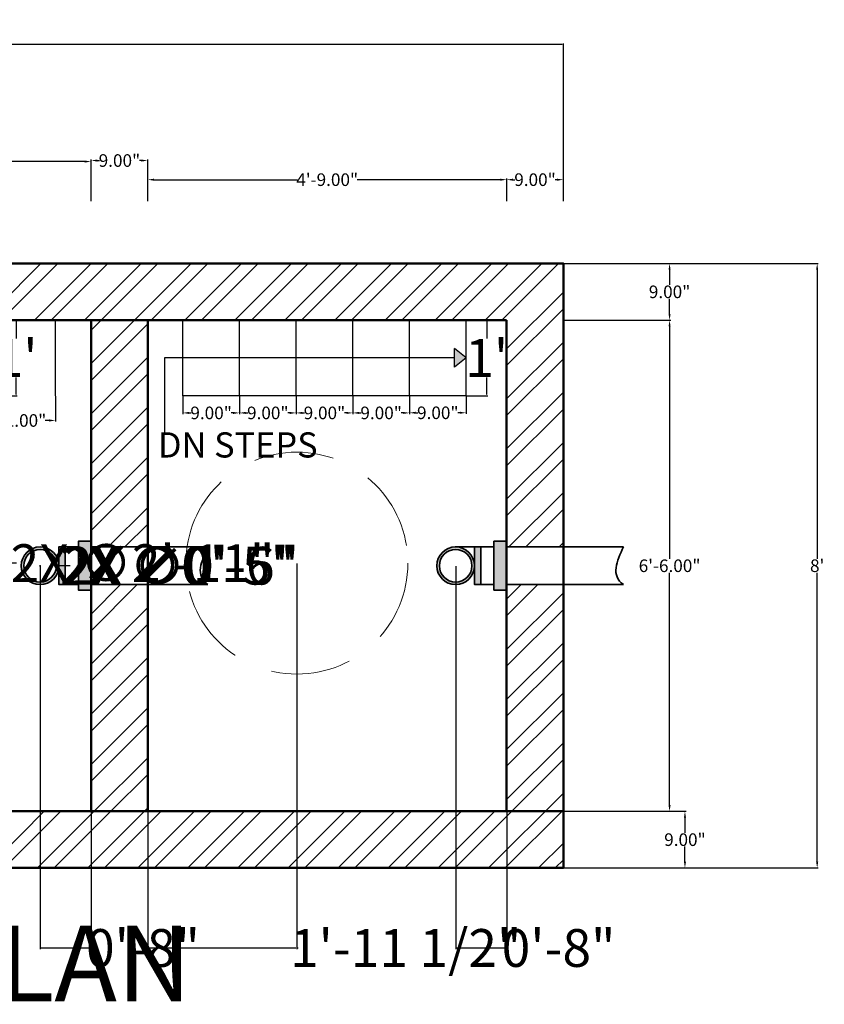
# Model space of a CAD drawing. Units: inches. Extents: x -34 to 285, y -151 to 155.
# Tile 10 of 10: x 129 to 256, y -2 to 155. Entities that reach past the tile are written whole.
import ezdxf

# ---------------------------------------------------------------- set-up
doc = ezdxf.new("R2010")
doc.units = ezdxf.units.IN
doc.header["$MEASUREMENT"] = 0
doc.linetypes.add('DASHED', pattern=[19.05, 12.7, -6.35])
for name, color, linetype, lineweight in [('A-ANNO-DIMS', 2, 'Continuous', 18), ('A-ANNO-TEXT', 7, 'Continuous', 25), ('A-DETL-HIDN', 8, 'DASHED', 18), ('A-FLOR-STRS', 3, 'Continuous', 25), ('A-WALL', 7, 'Continuous', 50), ('A-WALL-PATT', 8, 'Continuous', 18), ('P-SANR-PIPE', 4, 'Continuous', 35)]:
    doc.layers.add(name, color=color, linetype=linetype, lineweight=lineweight)
doc.styles.get("Standard").update_dxf_attribs({"font": 'arial.ttf'})
doc.dimstyles.get("Standard").update_dxf_attribs({"dimtxt": 6, "dimasz": 0.18, "dimexe": 0.18, "dimexo": 0.0625, "dimgap": 0.09, "dimtad": 0, "dimtih": 1, "dimtoh": 1, "dimzin": 0, "dimdsep": 46, "dimlunit": 3, "dimtxsty": 'Standard', "dimcen": 0.09, "dimadec": 0, "dimazin": 0, "dimtfac": 1, "dimtofl": 0, "dimtmove": 0, "dimatfit": 3, "dimfxl": 1, "dimtolj": 1, "dimtzin": 0, "dimarcsym": 0})

# ---------------------------------------------------------------- blocks, each defined once
blk = doc.blocks.new('*D1')
at = {"layer": 'A-ANNO-DIMS', "color": 0, "lineweight": -2, "transparency": 16777216}
for p, q in [((199.47, 106.98), (202.86, 106.98)), ((202.68, 106.8), (202.68, 104.08)), ((202.68, 95.16), (202.68, 97.88)), ((199.47, 94.98), (202.86, 94.98))]:
    blk.add_line(p, q, dxfattribs=at)
at = {"layer": 'A-ANNO-DIMS', "color": 0, "transparency": 16777216}
for points in [[(202.65, 106.8), (202.71, 106.8), (202.68, 106.98)], [(202.65, 95.16), (202.71, 95.16), (202.68, 94.98)]]:
    blk.add_solid(points, dxfattribs=at)
at = {"layer": 'Defpoints', "color": 0, "transparency": 16777216}
for p in [(199.41, 106.98), (199.41, 94.98), (202.68, 94.98)]:
    blk.add_point(p, dxfattribs=at)
at = {"layer": 'A-ANNO-DIMS', "color": 0, "transparency": 16777216, "insert": (202.68, 100.98), "char_height": 6, "attachment_point": 5}
blk.add_mtext("\\A1;1'", dxfattribs=at)
blk = doc.blocks.new('*D2')
at = {"layer": 'A-ANNO-DIMS', "color": 0, "lineweight": -2, "transparency": 16777216}
for p, q in [((190.41, 94.92), (190.41, 92.09)), ((199.41, 94.92), (199.41, 92.09)), ((191.41, 92.27), (191.73, 92.27)), ((198.41, 92.27), (198.09, 92.27))]:
    blk.add_line(p, q, dxfattribs=at)
at = {"layer": 'A-ANNO-DIMS', "color": 0, "transparency": 16777216}
for points in [[(191.41, 92.44), (191.41, 92.11), (190.41, 92.27)], [(198.41, 92.44), (198.41, 92.11), (199.41, 92.27)]]:
    blk.add_solid(points, dxfattribs=at)
at = {"layer": 'Defpoints', "color": 0, "transparency": 16777216}
for p in [(190.41, 94.98), (199.41, 94.98), (199.41, 92.27)]:
    blk.add_point(p, dxfattribs=at)
at = {"layer": 'A-ANNO-DIMS', "color": 0, "transparency": 16777216, "insert": (194.91, 92.27), "char_height": 2, "attachment_point": 5}
blk.add_mtext('\\A1;9.00"', dxfattribs=at)
blk = doc.blocks.new('*D3')
at = {"layer": 'A-ANNO-DIMS', "color": 0, "lineweight": -2, "transparency": 16777216}
for p, q in [((181.41, 94.92), (181.41, 92.07)), ((190.41, 94.92), (190.41, 92.07)), ((182.41, 92.25), (182.73, 92.25)), ((189.41, 92.25), (189.09, 92.25))]:
    blk.add_line(p, q, dxfattribs=at)
at = {"layer": 'A-ANNO-DIMS', "color": 0, "transparency": 16777216}
for points in [[(182.41, 92.41), (182.41, 92.08), (181.41, 92.25)], [(189.41, 92.41), (189.41, 92.08), (190.41, 92.25)]]:
    blk.add_solid(points, dxfattribs=at)
at = {"layer": 'Defpoints', "color": 0, "transparency": 16777216}
for p in [(181.41, 94.98), (190.41, 94.98), (181.41, 92.25)]:
    blk.add_point(p, dxfattribs=at)
at = {"layer": 'A-ANNO-DIMS', "color": 0, "transparency": 16777216, "insert": (185.91, 92.25), "char_height": 2, "attachment_point": 5}
blk.add_mtext('\\A1;9.00"', dxfattribs=at)
blk = doc.blocks.new('*D4')
at = {"layer": 'A-ANNO-DIMS', "color": 0, "lineweight": -2, "transparency": 16777216}
for p, q in [((172.41, 94.92), (172.41, 92.07)), ((181.41, 94.92), (181.41, 92.07)), ((173.41, 92.25), (173.73, 92.25)), ((180.41, 92.25), (180.09, 92.25))]:
    blk.add_line(p, q, dxfattribs=at)
at = {"layer": 'A-ANNO-DIMS', "color": 0, "transparency": 16777216}
for points in [[(173.41, 92.41), (173.41, 92.08), (172.41, 92.25)], [(180.41, 92.41), (180.41, 92.08), (181.41, 92.25)]]:
    blk.add_solid(points, dxfattribs=at)
at = {"layer": 'Defpoints', "color": 0, "transparency": 16777216}
for p in [(172.41, 94.98), (181.41, 94.98), (172.41, 92.25)]:
    blk.add_point(p, dxfattribs=at)
at = {"layer": 'A-ANNO-DIMS', "color": 0, "transparency": 16777216, "insert": (176.91, 92.25), "char_height": 2, "attachment_point": 5}
blk.add_mtext('\\A1;9.00"', dxfattribs=at)
blk = doc.blocks.new('*D5')
at = {"layer": 'A-ANNO-DIMS', "color": 0, "lineweight": -2, "transparency": 16777216}
for p, q in [((163.41, 94.92), (163.41, 92.07)), ((172.41, 94.92), (172.41, 92.07)), ((164.41, 92.25), (164.73, 92.25)), ((171.41, 92.25), (171.09, 92.25))]:
    blk.add_line(p, q, dxfattribs=at)
at = {"layer": 'A-ANNO-DIMS', "color": 0, "transparency": 16777216}
for points in [[(164.41, 92.41), (164.41, 92.08), (163.41, 92.25)], [(171.41, 92.41), (171.41, 92.08), (172.41, 92.25)]]:
    blk.add_solid(points, dxfattribs=at)
at = {"layer": 'Defpoints', "color": 0, "transparency": 16777216}
for p in [(163.41, 94.98), (172.41, 94.98), (163.41, 92.25)]:
    blk.add_point(p, dxfattribs=at)
at = {"layer": 'A-ANNO-DIMS', "color": 0, "transparency": 16777216, "insert": (167.91, 92.25), "char_height": 2, "attachment_point": 5}
blk.add_mtext('\\A1;9.00"', dxfattribs=at)
blk = doc.blocks.new('*D6')
at = {"layer": 'A-ANNO-DIMS', "color": 0, "lineweight": -2, "transparency": 16777216}
for p, q in [((154.41, 94.92), (154.41, 92.07)), ((163.41, 94.92), (163.41, 92.07)), ((155.41, 92.25), (155.73, 92.25)), ((162.41, 92.25), (162.09, 92.25))]:
    blk.add_line(p, q, dxfattribs=at)
at = {"layer": 'A-ANNO-DIMS', "color": 0, "transparency": 16777216}
for points in [[(155.41, 92.41), (155.41, 92.08), (154.41, 92.25)], [(162.41, 92.41), (162.41, 92.08), (163.41, 92.25)]]:
    blk.add_solid(points, dxfattribs=at)
at = {"layer": 'Defpoints', "color": 0, "transparency": 16777216}
for p in [(154.41, 94.98), (163.41, 94.98), (154.41, 92.25)]:
    blk.add_point(p, dxfattribs=at)
at = {"layer": 'A-ANNO-DIMS', "color": 0, "transparency": 16777216, "insert": (158.91, 92.25), "char_height": 2, "attachment_point": 5}
blk.add_mtext('\\A1;9.00"', dxfattribs=at)
blk = doc.blocks.new('*D7')
at = {"layer": 'A-ANNO-DIMS', "color": 0, "lineweight": -2, "transparency": 16777216}
for p, q in [((123.25, 106.98), (128.12, 106.98)), ((127.94, 106.8), (127.94, 104.08)), ((127.94, 95.16), (127.94, 97.88)), ((123.25, 94.98), (128.12, 94.98))]:
    blk.add_line(p, q, dxfattribs=at)
at = {"layer": 'A-ANNO-DIMS', "color": 0, "transparency": 16777216}
for points in [[(127.91, 106.8), (127.97, 106.8), (127.94, 106.98)], [(127.91, 95.16), (127.97, 95.16), (127.94, 94.98)]]:
    blk.add_solid(points, dxfattribs=at)
at = {"layer": 'Defpoints', "color": 0, "transparency": 16777216}
for p in [(123.18, 106.98), (123.18, 94.98), (127.94, 94.98)]:
    blk.add_point(p, dxfattribs=at)
at = {"layer": 'A-ANNO-DIMS', "color": 0, "transparency": 16777216, "insert": (127.94, 100.98), "char_height": 6, "attachment_point": 5}
blk.add_mtext("\\A1;1'", dxfattribs=at)
blk = doc.blocks.new('*D13')
at = {"layer": 'A-ANNO-DIMS', "color": 0, "lineweight": -2, "transparency": 16777216}
for p, q in [((123.18, 94.92), (123.18, 90.87)), ((134.18, 94.92), (134.18, 90.87)), ((124.18, 91.05), (124.82, 91.05)), ((133.18, 91.05), (132.55, 91.05))]:
    blk.add_line(p, q, dxfattribs=at)
at = {"layer": 'A-ANNO-DIMS', "color": 0, "transparency": 16777216}
for points in [[(124.18, 91.22), (124.18, 90.88), (123.18, 91.05)], [(133.18, 91.22), (133.18, 90.88), (134.18, 91.05)]]:
    blk.add_solid(points, dxfattribs=at)
at = {"layer": 'Defpoints', "color": 0, "transparency": 16777216}
for p in [(123.18, 94.98), (134.18, 94.98), (134.18, 91.05)]:
    blk.add_point(p, dxfattribs=at)
at = {"layer": 'A-ANNO-DIMS', "color": 0, "transparency": 16777216, "insert": (128.68, 91.05), "char_height": 2, "attachment_point": 5}
blk.add_mtext('\\A1;11.00"', dxfattribs=at)
blk = doc.blocks.new('*D17')
at = {"layer": 'A-ANNO-DIMS', "color": 0, "lineweight": -2, "transparency": 16777216}
for p, q in [((70.85, 125.9), (70.85, 132.35)), ((71.85, 132.17), (100.66, 132.17)), ((138.85, 132.17), (110.04, 132.17)), ((139.85, 125.9), (139.85, 132.35))]:
    blk.add_line(p, q, dxfattribs=at)
at = {"layer": 'A-ANNO-DIMS', "color": 0, "transparency": 16777216}
for points in [[(71.85, 132.33), (71.85, 132), (70.85, 132.17)], [(138.85, 132.33), (138.85, 132), (139.85, 132.17)]]:
    blk.add_solid(points, dxfattribs=at)
at = {"layer": 'Defpoints', "color": 0, "transparency": 16777216}
for p in [(139.85, 132.17), (70.85, 125.83), (139.85, 125.83)]:
    blk.add_point(p, dxfattribs=at)
at = {"layer": 'A-ANNO-DIMS', "color": 0, "transparency": 16777216, "insert": (105.35, 132.17), "char_height": 2, "attachment_point": 5}
blk.add_mtext('\\A1;5\'-9.00"', dxfattribs=at)
blk = doc.blocks.new('*D18')
at = {"layer": 'A-ANNO-DIMS', "color": 0, "lineweight": -2, "transparency": 16777216}
for p, q in [((139.85, 125.9), (139.85, 132.51)), ((140.85, 132.33), (141.16, 132.33)), ((147.85, 132.33), (147.53, 132.33)), ((148.85, 125.9), (148.85, 132.51))]:
    blk.add_line(p, q, dxfattribs=at)
at = {"layer": 'A-ANNO-DIMS', "color": 0, "transparency": 16777216}
for points in [[(140.85, 132.49), (140.85, 132.16), (139.85, 132.33)], [(147.85, 132.49), (147.85, 132.16), (148.85, 132.33)]]:
    blk.add_solid(points, dxfattribs=at)
at = {"layer": 'Defpoints', "color": 0, "transparency": 16777216}
for p in [(148.85, 132.33), (139.85, 125.83), (148.85, 125.83)]:
    blk.add_point(p, dxfattribs=at)
at = {"layer": 'A-ANNO-DIMS', "color": 0, "transparency": 16777216, "insert": (144.35, 132.33), "char_height": 2, "attachment_point": 5}
blk.add_mtext('\\A1;9.00"', dxfattribs=at)
blk = doc.blocks.new('*D19')
at = {"layer": 'A-ANNO-DIMS', "color": 0, "lineweight": -2, "transparency": 16777216}
for p, q in [((148.85, 125.9), (148.85, 129.47)), ((149.85, 129.29), (172.62, 129.29)), ((204.85, 129.29), (182.08, 129.29)), ((205.85, 125.9), (205.85, 129.47))]:
    blk.add_line(p, q, dxfattribs=at)
at = {"layer": 'A-ANNO-DIMS', "color": 0, "transparency": 16777216}
for points in [[(149.85, 129.45), (149.85, 129.12), (148.85, 129.29)], [(204.85, 129.45), (204.85, 129.12), (205.85, 129.29)]]:
    blk.add_solid(points, dxfattribs=at)
at = {"layer": 'Defpoints', "color": 0, "transparency": 16777216}
for p in [(205.85, 129.29), (148.85, 125.83), (205.85, 125.83)]:
    blk.add_point(p, dxfattribs=at)
at = {"layer": 'A-ANNO-DIMS', "color": 0, "transparency": 16777216, "insert": (177.35, 129.29), "char_height": 2, "attachment_point": 5}
blk.add_mtext('\\A1;4\'-9.00"', dxfattribs=at)
blk = doc.blocks.new('*D20')
at = {"layer": 'A-ANNO-DIMS', "color": 0, "lineweight": -2, "transparency": 16777216}
for p, q in [((205.85, 125.9), (205.85, 129.47)), ((206.85, 129.29), (207.16, 129.29)), ((213.85, 129.29), (213.53, 129.29)), ((214.85, 125.9), (214.85, 129.47))]:
    blk.add_line(p, q, dxfattribs=at)
at = {"layer": 'A-ANNO-DIMS', "color": 0, "transparency": 16777216}
for points in [[(206.85, 129.45), (206.85, 129.12), (205.85, 129.29)], [(213.85, 129.45), (213.85, 129.12), (214.85, 129.29)]]:
    blk.add_solid(points, dxfattribs=at)
at = {"layer": 'Defpoints', "color": 0, "transparency": 16777216}
for p in [(214.85, 129.29), (205.85, 125.83), (214.85, 125.83)]:
    blk.add_point(p, dxfattribs=at)
at = {"layer": 'A-ANNO-DIMS', "color": 0, "transparency": 16777216, "insert": (210.35, 129.29), "char_height": 2, "attachment_point": 5}
blk.add_mtext('\\A1;9.00"', dxfattribs=at)
blk = doc.blocks.new('*D21')
at = {"layer": 'A-ANNO-DIMS', "color": 0, "lineweight": -2, "transparency": 16777216}
for p, q in [((22.85, 130.62), (22.85, 150.94)), ((23.03, 150.76), (113.95, 150.76)), ((214.67, 150.76), (123.74, 150.76)), ((214.85, 127.74), (214.85, 150.94))]:
    blk.add_line(p, q, dxfattribs=at)
at = {"layer": 'A-ANNO-DIMS', "color": 0, "transparency": 16777216}
for points in [[(23.03, 150.79), (23.03, 150.73), (22.85, 150.76)], [(214.67, 150.79), (214.67, 150.73), (214.85, 150.76)]]:
    blk.add_solid(points, dxfattribs=at)
at = {"layer": 'Defpoints', "color": 0, "transparency": 16777216}
for p in [(22.85, 150.76), (22.85, 130.55), (214.85, 127.68)]:
    blk.add_point(p, dxfattribs=at)
at = {"layer": 'A-ANNO-DIMS', "color": 0, "transparency": 16777216, "insert": (118.85, 150.76), "char_height": 6, "attachment_point": 5}
blk.add_mtext("\\A1;16'", dxfattribs=at)
blk = doc.blocks.new('*D22')
at = {"layer": 'A-ANNO-DIMS', "color": 0, "lineweight": -2, "transparency": 16777216}
for p, q in [((214.91, 115.98), (231.9, 115.98)), ((231.72, 114.98), (231.72, 112.59)), ((231.72, 107.98), (231.72, 110.37)), ((214.91, 106.98), (231.9, 106.98))]:
    blk.add_line(p, q, dxfattribs=at)
at = {"layer": 'A-ANNO-DIMS', "color": 0, "transparency": 16777216}
for points in [[(231.55, 114.98), (231.88, 114.98), (231.72, 115.98)], [(231.55, 107.98), (231.88, 107.98), (231.72, 106.98)]]:
    blk.add_solid(points, dxfattribs=at)
at = {"layer": 'Defpoints', "color": 0, "transparency": 16777216}
for p in [(214.85, 115.98), (231.72, 115.98), (214.85, 106.98)]:
    blk.add_point(p, dxfattribs=at)
at = {"layer": 'A-ANNO-DIMS', "color": 0, "transparency": 16777216, "insert": (231.72, 111.48), "char_height": 2, "attachment_point": 5}
blk.add_mtext('\\A1;9.00"', dxfattribs=at)
blk = doc.blocks.new('*D23')
at = {"layer": 'A-ANNO-DIMS', "color": 0, "lineweight": -2, "transparency": 16777216}
for p, q in [((214.91, 28.98), (234.34, 28.98)), ((234.16, 27.98), (234.16, 25.59)), ((234.16, 20.98), (234.16, 23.37)), ((214.91, 19.98), (234.34, 19.98))]:
    blk.add_line(p, q, dxfattribs=at)
at = {"layer": 'A-ANNO-DIMS', "color": 0, "transparency": 16777216}
for points in [[(234, 27.98), (234.33, 27.98), (234.16, 28.98)], [(234, 20.98), (234.33, 20.98), (234.16, 19.98)]]:
    blk.add_solid(points, dxfattribs=at)
at = {"layer": 'Defpoints', "color": 0, "transparency": 16777216}
for p in [(214.85, 28.98), (214.85, 19.98), (234.16, 19.98)]:
    blk.add_point(p, dxfattribs=at)
at = {"layer": 'A-ANNO-DIMS', "color": 0, "transparency": 16777216, "insert": (234.16, 24.48), "char_height": 2, "attachment_point": 5}
blk.add_mtext('\\A1;9.00"', dxfattribs=at)
blk = doc.blocks.new('*D24')
at = {"layer": 'A-ANNO-DIMS', "color": 0, "lineweight": -2, "transparency": 16777216}
for p, q in [((231.78, 106.98), (231.9, 106.98)), ((231.72, 105.98), (231.72, 69.09)), ((231.72, 29.98), (231.72, 66.87)), ((231.78, 28.98), (231.9, 28.98))]:
    blk.add_line(p, q, dxfattribs=at)
at = {"layer": 'A-ANNO-DIMS', "color": 0, "transparency": 16777216}
for points in [[(231.55, 105.98), (231.88, 105.98), (231.72, 106.98)], [(231.55, 29.98), (231.88, 29.98), (231.72, 28.98)]]:
    blk.add_solid(points, dxfattribs=at)
at = {"layer": 'Defpoints', "color": 0, "transparency": 16777216}
for p in [(231.72, 106.98), (231.72, 28.98), (231.72, 28.98)]:
    blk.add_point(p, dxfattribs=at)
at = {"layer": 'A-ANNO-DIMS', "color": 0, "transparency": 16777216, "insert": (231.72, 67.98), "char_height": 2, "attachment_point": 5}
blk.add_mtext('\\A1;6\'-6.00"', dxfattribs=at)
blk = doc.blocks.new('*D25')
at = {"layer": 'A-ANNO-DIMS', "color": 0, "lineweight": -2, "transparency": 16777216}
for p, q in [((231.96, 115.98), (255.34, 115.98)), ((255.16, 114.98), (255.16, 69.09)), ((255.16, 20.98), (255.16, 66.87)), ((231.78, 19.98), (255.34, 19.98))]:
    blk.add_line(p, q, dxfattribs=at)
at = {"layer": 'A-ANNO-DIMS', "color": 0, "transparency": 16777216}
for points in [[(254.99, 114.98), (255.32, 114.98), (255.16, 115.98)], [(254.99, 20.98), (255.32, 20.98), (255.16, 19.98)]]:
    blk.add_solid(points, dxfattribs=at)
at = {"layer": 'Defpoints', "color": 0, "transparency": 16777216}
for p in [(231.9, 115.98), (255.16, 115.98), (231.72, 19.98)]:
    blk.add_point(p, dxfattribs=at)
at = {"layer": 'A-ANNO-DIMS', "color": 0, "transparency": 16777216, "insert": (255.16, 67.98), "char_height": 2, "attachment_point": 5}
blk.add_mtext("\\A1;8'", dxfattribs=at)
blk = doc.blocks.new('PIPE-BEND-PLAN')
h = blk.add_hatch(color=256)
h.dxf.hatch_style = 1
h.paths.add_polyline_path([(3.06, 6.87), (2.93, 6.87, 0.408167), (0, 3.87, 1), (5.99, 3.87, 0.408167)])
h.paths.add_polyline_path([(5.59, 3.87, -1), (0.4, 3.87, -1)], flags=16)
h = blk.add_hatch(color=256)
h.dxf.hatch_style = 1
h.paths.add_polyline_path([(6.97, 6.87), (5.99, 6.87), (5.99, 0.87), (6.97, 0.87)])
h = blk.add_hatch(color=256)
h.dxf.hatch_style = 1
h.paths.add_polyline_path([(11.09, 7.75), (9.08, 7.75), (9.08, 0), (11.09, 0)])
for points in [[(6.97, 6.88), (5.99, 6.88), (5.99, 0.87), (6.97, 0.87)], [(9.08, 6.88), (6.97, 6.88), (6.97, 0.87), (9.08, 0.87)], [(11.09, 7.75), (9.08, 7.75), (9.08, 0), (11.09, 0)]]:
    blk.add_lwpolyline(points, close=True)
for radius in [2.99, 2.59]:
    blk.add_circle((2.99, 3.87), radius)
blk = doc.blocks.new('*D41')
at = {"layer": 'A-ANNO-DIMS', "color": 0, "lineweight": -2, "transparency": 16777216}
for p, q in [((172.53, 68.33), (172.53, 7.1)), ((148.85, 28.92), (148.85, 7.1)), ((149.03, 7.28), (172.35, 7.28)), ((172.53, 7.28), (172.71, 7.28))]:
    blk.add_line(p, q, dxfattribs=at)
at = {"layer": 'A-ANNO-DIMS', "color": 0, "transparency": 16777216}
for points in [[(149.03, 7.31), (149.03, 7.25), (148.85, 7.28)], [(172.35, 7.31), (172.35, 7.25), (172.53, 7.28)]]:
    blk.add_solid(points, dxfattribs=at)
at = {"layer": 'Defpoints', "color": 0, "transparency": 16777216}
for p in [(172.53, 68.39), (148.85, 28.98), (172.53, 7.28)]:
    blk.add_point(p, dxfattribs=at)
at = {"layer": 'A-ANNO-DIMS', "color": 0, "transparency": 16777216, "insert": (189.81, 7.28), "char_height": 6, "attachment_point": 5}
blk.add_mtext('\\A1;1\'-11 1/2"', dxfattribs=at)
blk = doc.blocks.new('*D44')
at = {"layer": 'A-ANNO-DIMS', "color": 0, "lineweight": -2, "transparency": 16777216}
for p, q in [((131.75, 67.92), (131.75, 7.1)), ((139.85, 28.92), (139.85, 7.1)), ((131.93, 7.28), (139.67, 7.28)), ((139.85, 7.28), (140.03, 7.28))]:
    blk.add_line(p, q, dxfattribs=at)
at = {"layer": 'A-ANNO-DIMS', "color": 0, "transparency": 16777216}
for points in [[(131.93, 7.31), (131.93, 7.25), (131.75, 7.28)], [(139.67, 7.31), (139.67, 7.25), (139.85, 7.28)]]:
    blk.add_solid(points, dxfattribs=at)
at = {"layer": 'Defpoints', "color": 0, "transparency": 16777216}
for p in [(131.75, 67.99), (139.85, 28.98), (139.85, 7.28)]:
    blk.add_point(p, dxfattribs=at)
at = {"layer": 'A-ANNO-DIMS', "color": 0, "transparency": 16777216, "insert": (148.09, 7.28), "char_height": 6, "attachment_point": 5}
blk.add_mtext('\\A1;0\'-8"', dxfattribs=at)
blk = doc.blocks.new('*D45')
at = {"layer": 'A-ANNO-DIMS', "color": 0, "lineweight": -2, "transparency": 16777216}
for p, q in [((197.75, 67.92), (197.75, 7.1)), ((205.85, 28.92), (205.85, 7.1)), ((197.93, 7.28), (205.67, 7.28)), ((205.85, 7.28), (206.03, 7.28))]:
    blk.add_line(p, q, dxfattribs=at)
at = {"layer": 'A-ANNO-DIMS', "color": 0, "transparency": 16777216}
for points in [[(197.93, 7.31), (197.93, 7.25), (197.75, 7.28)], [(205.67, 7.31), (205.67, 7.25), (205.85, 7.28)]]:
    blk.add_solid(points, dxfattribs=at)
at = {"layer": 'Defpoints', "color": 0, "transparency": 16777216}
for p in [(197.75, 67.99), (205.85, 28.98), (205.85, 7.28)]:
    blk.add_point(p, dxfattribs=at)
at = {"layer": 'A-ANNO-DIMS', "color": 0, "transparency": 16777216, "insert": (214.09, 7.28), "char_height": 6, "attachment_point": 5}
blk.add_mtext('\\A1;0\'-8"', dxfattribs=at)
blk = doc.blocks.new('*D88')
at = {"layer": 'A-ANNO-DIMS', "color": 0, "lineweight": -2, "transparency": 16777216}
for p, q in [((99.72, 68.39), (99.9, 68.39)), ((99.81, 68.3), (99.81, 68.48)), ((128.01, 68.39), (117.62, 68.39))]:
    blk.add_line(p, q, dxfattribs=at)
at = {"layer": 'A-ANNO-DIMS', "color": 0, "transparency": 16777216}
blk.add_solid([(117.62, 68.42), (117.62, 68.36), (117.44, 68.39)], dxfattribs=at)
at = {"layer": 'Defpoints', "color": 0, "transparency": 16777216}
for p in [(82.19, 68.39), (117.44, 68.39)]:
    blk.add_point(p, dxfattribs=at)
at = {"layer": 'A-ANNO-DIMS', "color": 0, "transparency": 16777216, "insert": (148.01, 68.39), "char_height": 6, "attachment_point": 5}
blk.add_mtext('\\A1;2X ∅2\'-11"', dxfattribs=at)
blk = doc.blocks.new('*D91')
at = {"layer": 'A-ANNO-DIMS', "color": 0, "lineweight": -2, "transparency": 16777216}
for p, q in [((131.66, 67.99), (131.84, 67.99)), ((131.75, 67.9), (131.75, 68.08)), ((136.54, 67.99), (134.92, 67.99))]:
    blk.add_line(p, q, dxfattribs=at)
at = {"layer": 'A-ANNO-DIMS', "color": 0, "transparency": 16777216}
blk.add_solid([(134.92, 68.02), (134.92, 67.96), (134.74, 67.99)], dxfattribs=at)
at = {"layer": 'Defpoints', "color": 0, "transparency": 16777216}
for p in [(128.75, 67.99), (134.74, 67.99)]:
    blk.add_point(p, dxfattribs=at)
at = {"layer": 'A-ANNO-DIMS', "color": 0, "transparency": 16777216, "insert": (154.21, 67.99), "char_height": 6, "attachment_point": 5}
blk.add_mtext('\\A1;2X ∅0\'-6"', dxfattribs=at)
blk = doc.blocks.new('*D92')
at = {"layer": 'A-ANNO-DIMS', "color": 0, "lineweight": -2, "transparency": 16777216}
for p, q in [((131.66, 67.99), (131.84, 67.99)), ((131.75, 67.9), (131.75, 68.08)), ((135.9, 67.99), (134.52, 67.99))]:
    blk.add_line(p, q, dxfattribs=at)
at = {"layer": 'A-ANNO-DIMS', "color": 0, "transparency": 16777216}
blk.add_solid([(134.52, 68.02), (134.52, 67.96), (134.34, 67.99)], dxfattribs=at)
at = {"layer": 'Defpoints', "color": 0, "transparency": 16777216}
for p in [(129.15, 67.99), (134.34, 67.99)]:
    blk.add_point(p, dxfattribs=at)
at = {"layer": 'A-ANNO-DIMS', "color": 0, "transparency": 16777216, "insert": (153.57, 67.99), "char_height": 6, "attachment_point": 5}
blk.add_mtext('\\A1;2X ∅0\'-5"', dxfattribs=at)

msp = doc.modelspace()

# ---------------------------------------------------------------- hatches: boundary and pattern name
at = {"layer": 'A-FLOR-STRS'}
h = msp.add_hatch(color=256, dxfattribs=at)
h.dxf.hatch_style = 1
h.paths.add_polyline_path([(197.548, 102.473), (197.539, 99.493), (199.408, 100.981)])
at = {"layer": 'A-WALL-PATT'}
h = msp.add_hatch(dxfattribs=at)
h.set_pattern_fill('ANSI32', color=256, scale=15)
h.paths.add_polyline_path([(214.846, 64.981), (205.846, 64.981), (205.846, 64.112), (205.846, 28.981), (31.846, 28.981), (31.846, 64.981), (22.846, 64.981), (22.846, 19.981), (214.846, 19.981)])
h.paths.add_polyline_path([(67.846, 106.981), (67.846, 115.981), (22.846, 115.981), (22.846, 70.981), (31.846, 70.981), (31.846, 106.981)])
h = msp.add_hatch(dxfattribs=at)
h.set_pattern_fill('ANSI32', color=256, scale=15)
h.paths.add_polyline_path([(214.846, 115.981), (22.846, 115.981), (22.846, 70.981), (31.846, 70.981), (31.846, 106.981), (205.846, 106.981), (205.846, 70.981), (214.846, 70.981)])
h = msp.add_hatch(dxfattribs=at)
h.set_pattern_fill('ANSI32', color=256, scale=15)
h.paths.add_polyline_path([(139.846, 70.981), (148.846, 70.981), (148.846, 106.981), (139.846, 106.981)])
h.paths.add_polyline_path([(148.846, 64.981), (139.846, 64.981), (139.846, 64.112), (139.846, 28.981), (148.846, 28.981)])

# ---------------------------------------------------------------- linework, layer by layer
at = {"layer": 'A-DETL-HIDN'}
msp.add_circle((172.528, 68.391), 17.624, dxfattribs=at)
at = {"layer": 'A-FLOR-STRS'}
for p, q in [((134.184, 94.981), (134.184, 106.981)), ((154.408, 94.981), (154.408, 106.981)), ((163.408, 94.981), (163.408, 106.981)), ((172.408, 94.981), (172.408, 106.981)), ((181.408, 94.981), (181.408, 106.981)), ((190.408, 94.981), (190.408, 106.981)), ((199.408, 94.981), (199.408, 106.981)), ((197.539, 99.493), (197.548, 102.473)), ((199.408, 100.981), (197.548, 102.473)), ((197.544, 100.981), (151.489, 100.981)), ((151.489, 100.981), (151.489, 89.167)), ((199.408, 100.981), (197.539, 99.493))]:
    msp.add_line(p, q, dxfattribs=at)
msp.add_lwpolyline([(199.408, 94.981), (154.408, 94.981)], dxfattribs=at)
at = {"layer": 'A-WALL'}
for points in [[(22.846, 64.981), (22.846, 19.981), (214.846, 19.981), (214.846, 115.981), (22.846, 115.981), (22.846, 70.981)], [(205.846, 106.981), (31.846, 106.981)], [(139.846, 106.981), (139.846, 28.981)], [(148.846, 106.981), (148.846, 28.981)], [(205.846, 28.981), (205.846, 106.981)], [(31.846, 28.981), (214.846, 28.981)]]:
    msp.add_lwpolyline(points, dxfattribs=at)
at = {"layer": 'P-SANR-PIPE'}
for p, q in [((139.846, 70.981), (158.397, 70.981)), ((139.846, 70.981), (148.846, 70.981)), ((197.687, 70.981), (203.829, 70.981)), ((205.846, 70.981), (214.846, 70.981)), ((139.846, 64.981), (158.397, 64.981)), ((139.846, 64.981), (148.846, 64.981)), ((200.743, 64.981), (203.829, 64.981)), ((205.846, 64.981), (214.846, 64.981))]:
    msp.add_line(p, q, dxfattribs=at)
for points in [[(149.122, 64.981), (139.846, 64.981), (139.846, 70.981), (149.122, 70.981)], [(158.397, 64.981), (148.846, 64.981), (148.846, 70.981), (158.397, 70.981)], [(224.397, 64.981), (214.846, 64.981), (214.846, 70.981), (224.397, 70.981)]]:
    msp.add_lwpolyline(points, dxfattribs=at)
msp.add_lwpolyline([(139.846, 70.981), (148.846, 70.981), (148.846, 64.981), (139.846, 64.981)], close=True, dxfattribs=at)
for points in [[(158.397, 70.981), (157.356, 68.695), (156.314, 66.41), (158.397, 64.981)], [(224.397, 70.981), (223.356, 68.695), (222.314, 66.41), (224.397, 64.981)]]:
    msp.add_open_spline(points, degree=3, dxfattribs=at)

# ---------------------------------------------------------------- block references
for p in [(128.754, 64.112), (194.754, 64.112)]:
    msp.add_blockref('PIPE-BEND-PLAN', p, dxfattribs=at)

# ---------------------------------------------------------------- texts
at = {"layer": 'A-ANNO-TEXT', "attachment_point": 1}
for s, insert, char_height in [('DN STEPS', (150.461, 89.167), 4), ('PLAN ', (114.748, 10.798), 12)]:
    msp.add_mtext_dynamic_manual_height_columns(s, width=53.60251, gutter_width=1, heights=[0], dxfattribs=dict(at, insert=insert, char_height=char_height))

# ---------------------------------------------------------------- dimensions: what is measured, and where the dimension line sits
at = {"layer": 'A-ANNO-DIMS'}
for base, p1, p2, override, picture, middle in [((22.846, 150.759), (214.846, 127.681), (22.846, 130.553), {"dimclrd": 0, "dimclre": 0, "dimclrt": 0}, '*D21', (118.846, 150.759)), ((139.846, 132.167), (70.846, 125.833), (139.846, 125.833), {"dimtxt": 2, "dimasz": 1, "dimclrd": 0, "dimclre": 0, "dimclrt": 0}, '*D17', (105.346, 132.167)), ((148.846, 132.326), (139.846, 125.833), (148.846, 125.833), {"dimtxt": 2, "dimasz": 1, "dimclrd": 0, "dimclre": 0, "dimclrt": 0}, '*D18', (144.346, 132.326)), ((205.846, 129.287), (148.846, 125.833), (205.846, 125.833), {"dimtxt": 2, "dimasz": 1, "dimclrd": 0, "dimclre": 0, "dimclrt": 0}, '*D19', (177.346, 129.287)), ((214.846, 129.287), (205.846, 125.833), (214.846, 125.833), {"dimtxt": 2, "dimasz": 1, "dimclrd": 0, "dimclre": 0, "dimclrt": 0}, '*D20', (210.346, 129.287)), ((134.184, 91.051), (123.184, 94.981), (134.184, 94.981), {"dimtxt": 2, "dimasz": 1, "dimclrd": 0, "dimclre": 0, "dimclrt": 0}, '*D13', (128.684, 91.051)), ((154.408, 92.248), (163.408, 94.981), (154.408, 94.981), {"dimtxt": 2, "dimasz": 1, "dimclrd": 0, "dimclre": 0, "dimclrt": 0}, '*D6', (158.908, 92.248)), ((163.408, 92.248), (172.408, 94.981), (163.408, 94.981), {"dimtxt": 2, "dimasz": 1, "dimclrd": 0, "dimclre": 0, "dimclrt": 0}, '*D5', (167.908, 92.248)), ((172.408, 92.248), (181.408, 94.981), (172.408, 94.981), {"dimtxt": 2, "dimasz": 1, "dimclrd": 0, "dimclre": 0, "dimclrt": 0}, '*D4', (176.908, 92.248)), ((181.408, 92.248), (190.408, 94.981), (181.408, 94.981), {"dimtxt": 2, "dimasz": 1, "dimclrd": 0, "dimclre": 0, "dimclrt": 0}, '*D3', (185.908, 92.248)), ((199.408, 92.275), (190.408, 94.981), (199.408, 94.981), {"dimtxt": 2, "dimasz": 1, "dimclrd": 0, "dimclre": 0, "dimclrt": 0}, '*D2', (194.908, 92.275)), ((139.846, 7.281), (131.749, 67.987), (139.846, 28.981), {"dimdec": 1, "dimlfac": 1, "dimrnd": 0, "dimzin": 1, "dimdsep": 46, "dimlunit": 4, "dimfrac": 2}, '*D44', (148.091, 7.281)), ((172.528, 7.281), (148.846, 28.981), (172.528, 68.391), {"dimdec": 1, "dimlfac": 1, "dimrnd": 0, "dimzin": 1, "dimdsep": 46, "dimlunit": 4, "dimfrac": 2}, '*D41', (189.812, 7.281)), ((205.846, 7.281), (197.749, 67.987), (205.846, 28.981), {"dimdec": 1, "dimlfac": 1, "dimrnd": 0, "dimzin": 1, "dimdsep": 46, "dimlunit": 4, "dimfrac": 2}, '*D45', (214.091, 7.281))]:
    dim = msp.add_linear_dim(base=base, p1=p1, p2=p2, dimstyle='Standard', override=override, dxfattribs=at)
    dim.commit()
    dim.dimension.update_dxf_attribs({"geometry": picture, "text_midpoint": middle})
for base, p1, p2, override, picture, middle in [((231.715, 115.981), (214.846, 106.981), (214.846, 115.981), {"dimtxt": 2, "dimasz": 1, "dimclrd": 0, "dimclre": 0, "dimclrt": 0}, '*D22', (231.715, 111.481)), ((255.156, 115.981), (231.715, 19.981), (231.895, 115.981), {"dimtxt": 2, "dimasz": 1, "dimclrd": 0, "dimclre": 0, "dimclrt": 0}, '*D25', (255.156, 67.981)), ((127.945, 94.981), (123.184, 106.981), (123.184, 94.981), {"dimclrd": 0, "dimclre": 0, "dimclrt": 0}, '*D7', (127.945, 100.981)), ((202.677, 94.981), (199.408, 106.981), (199.408, 94.981), {"dimclrd": 0, "dimclre": 0, "dimclrt": 0}, '*D1', (202.677, 100.981)), ((231.715, 28.981), (231.715, 106.981), (231.715, 28.981), {"dimtxt": 2, "dimasz": 1, "dimclrd": 0, "dimclre": 0, "dimclrt": 0}, '*D24', (231.715, 67.981)), ((234.164, 19.981), (214.846, 28.981), (214.846, 19.981), {"dimtxt": 2, "dimasz": 1, "dimclrd": 0, "dimclre": 0, "dimclrt": 0}, '*D23', (234.164, 24.481))]:
    dim = msp.add_linear_dim(base=base, p1=p1, p2=p2, angle=90, dimstyle='Standard', override=override, dxfattribs=at)
    dim.commit()
    dim.dimension.update_dxf_attribs({"geometry": picture, "text_midpoint": middle})
for p1, p2, picture, middle in [((82.19, 68.39), (117.439, 68.391), '*D88', (128.013, 68.391)), ((128.754, 67.987), (134.743, 67.987), '*D91', (136.54, 67.987)), ((129.154, 67.987), (134.343, 67.987), '*D92', (135.9, 67.987))]:
    dim = msp.add_diameter_dim_2p(p1=p1, p2=p2, text='2X <>', dimstyle='Standard', override={"dimdec": 1, "dimlfac": 1, "dimrnd": 0, "dimzin": 1, "dimdsep": 46, "dimlunit": 4, "dimfrac": 2}, dxfattribs=at)
    dim.commit()
    dim.dimension.update_dxf_attribs({"geometry": picture, "text_midpoint": middle, "dimtype": 163})

doc.saveas('drawing.dxf')
